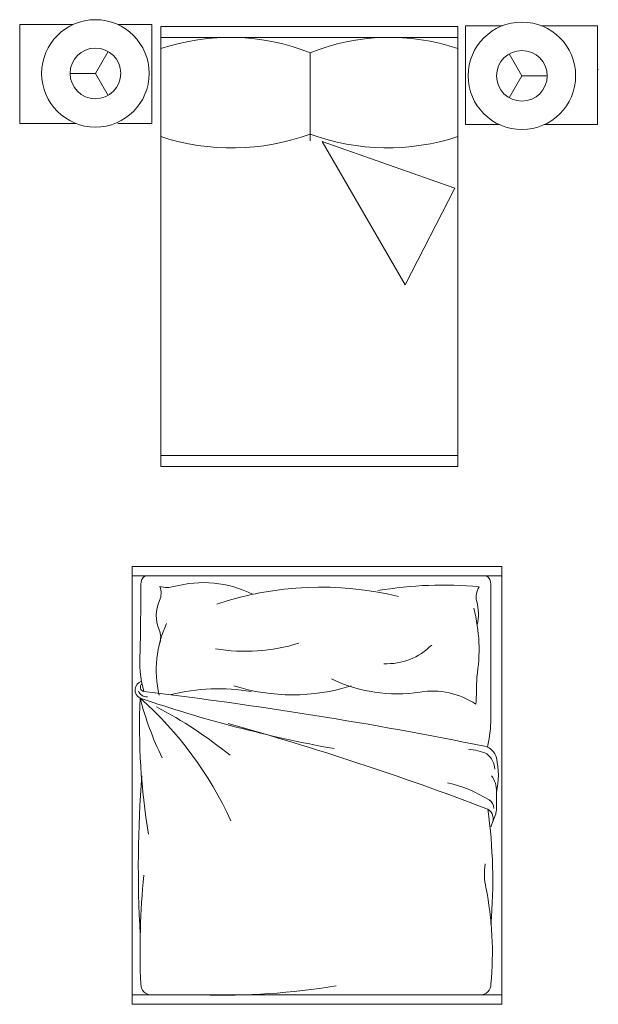
# Model space of a CAD drawing. Units: inches. Extents: x 1994 to 3075, y 3517 to 3950.
# Tile 10 of 58: x 1994.1175 to 1994.221, y 3553.7079 to 3553.8842. Entities that reach past the tile are written whole.
import ezdxf

# ---------------------------------------------------------------- set-up
doc = ezdxf.new("R2010")
doc.units = ezdxf.units.IN
doc.layers.add('A-FURN-REFR', color=8, linetype='Continuous', lineweight=13)

msp = doc.modelspace()

# ---------------------------------------------------------------- linework, layer by layer
at = {"layer": 'A-FURN-REFR'}
for p, q in [((1994.117509432348, 3553.883333005121), (1994.117509432348, 3553.865616469688)), ((1994.127049437094, 3553.883333005121), (1994.117509432348, 3553.883333005121)), ((1994.141131479592, 3553.883333005121), (1994.135063195254, 3553.883333005121)), ((1994.141131479592, 3553.883333005121), (1994.141131479592, 3553.865616469688)), ((1994.142742782828, 3553.804228108823), (1994.142742782828, 3553.882968266304)), ((1994.195892389127, 3553.882968266304), (1994.142742782828, 3553.882968266304)), ((1994.195892389127, 3553.804228108823), (1994.195892389127, 3553.882968266304)), ((1994.19728760273, 3553.865416846483), (1994.19728760273, 3553.883133381916)), ((1994.19728760273, 3553.883133381916), (1994.203900343284, 3553.883133381916)), ((1994.210825189012, 3553.883133381916), (1994.220909649974, 3553.883133381916)), ((1994.220909649974, 3553.865416846483), (1994.220909649974, 3553.883133381916)), ((1994.195892389127, 3553.880999762367), (1994.142742782828, 3553.880999762367)), ((1994.131056316174, 3553.874589508938), (1994.133323201859, 3553.878515870119)), ((1994.169474900446, 3553.862532974195), (1994.169474900446, 3553.878281005691)), ((1994.207362766148, 3553.874160342666), (1994.205095880463, 3553.878086703847)), ((1994.221034633952, 3553.875241371727), (1994.220909649974, 3553.875366355705)), ((1994.131056316174, 3553.874589508938), (1994.126522544804, 3553.874589508938)), ((1994.131056316174, 3553.874589508938), (1994.133323201859, 3553.870663147756)), ((1994.207362766148, 3553.874160342666), (1994.205095880463, 3553.870233981485)), ((1994.207362766148, 3553.874160342666), (1994.211896537518, 3553.874160342666)), ((1994.12759389331, 3553.865616469688), (1994.117509432348, 3553.865616469688)), ((1994.141131479592, 3553.865616469688), (1994.135063195254, 3553.865616469688)), ((1994.19728760273, 3553.865416846483), (1994.203355887068, 3553.865416846483)), ((1994.211369645228, 3553.865416846483), (1994.220909649974, 3553.865416846483)), ((1994.195360842532, 3553.854041419548), (1994.171645162721, 3553.862373044578)), ((1994.186492509023, 3553.836735927227), (1994.171645162721, 3553.862373044578)), ((1994.195360842532, 3553.854041419548), (1994.186492509023, 3553.836735927227)), ((1994.195892389127, 3553.80619661276), (1994.142742782828, 3553.80619661276)), ((1994.195892389127, 3553.804228108823), (1994.142742782828, 3553.804228108823)), ((1994.13761850143, 3553.786327657019), (1994.203768317831, 3553.786327657006)), ((1994.13761850143, 3553.786327657019), (1994.137618501414, 3553.707920668756)), ((1994.203768317831, 3553.786327657006), (1994.203768317815, 3553.707920668742)), ((1994.137618501429, 3553.784654455781), (1994.20376831783, 3553.784654455768)), ((1994.20182273499, 3553.759147087566), (1994.201822734995, 3553.783097989499)), ((1994.202795526404, 3553.742699450552), (1994.202795526405, 3553.746517277539)), ((1994.202675320726, 3553.742026181805), (1994.201822734986, 3553.739714637505)), ((1994.137618501414, 3553.709593869994), (1994.203768317815, 3553.709593869981)), ((1994.137618501414, 3553.707920668756), (1994.203768317815, 3553.707920668742))]:
    msp.add_line(p, q, dxfattribs=at)
for centre, radius in [((1994.131056316174, 3553.874589508938), 0.0096178898656984), ((1994.207362766148, 3553.874160342666), 0.0096178898656984), ((1994.131056316174, 3553.874589508938), 0.004533771369707), ((1994.207362766148, 3553.874160342666), 0.004533771369707)]:
    msp.add_circle(centre, radius, dxfattribs=at)
for centre, radius, start, end in [((1994.155078837424, 3553.84195624103), 0.0390734584879713, 68.38081539171897, 108.4039485392068), ((1994.183695872419, 3553.843014126873), 0.0380261592246056, 71.29230697710972, 111.9612016907544), ((1994.15550083672, 3553.902282602643), 0.0410331481229022, 251.8852769299205, 289.9107209210493), ((1994.183286182339, 3553.901481352651), 0.0402245355213375, 249.9186093217453, 288.2640062866705), ((1994.141120550532, 3553.783097989512), 0.0019455828353276, 126.8698976337993, 179.9999999880876), ((1994.19987715216, 3553.7830979895), 0.0019455828353276, 359.9999999880876, 53.13010234330246), ((1993.601556575717, 3553.782256987198), 0.5376190497749752, 358.8114973710085, 0.0896283401223897), ((1994.139610526882, 3553.781527333681), 0.0032028341489732, 335.7877323280015, 21.71237864400314), ((1994.143846681053, 3553.787202677152), 0.0046640380554646, 254.3196277006035, 285.6803722997152), ((1994.1503379227, 3553.763668816497), 0.0197486987265365, 63.38196750841395, 105.3587807882128), ((1994.171396254335, 3553.723937389351), 0.0586716085832465, 76.33335198625635, 108.4694926903225), ((1994.193173667668, 3553.714879910245), 0.0680947404926167, 84.45870901972506, 99.7951687550354), ((1994.202275155399, 3553.780846544132), 0.0031075126812102, 144.3787648229011, 195.1987658355305), ((1994.148529566308, 3553.777516662834), 0.0065764677133891, 155.7877323280015, 202.8808293159797), ((1994.169841135078, 3553.771464333994), 0.0298558147000044, 350.3711224665587, 14.25995084780135), ((1994.190980737527, 3553.777778179954), 0.0085962787467616, 347.311957921453, 15.19876583553051), ((1994.161796708111, 3553.767753433195), 0.0198519972069101, 155.1179531461462, 192.9861889591517), ((1994.139393198019, 3553.773660911681), 0.0033401870886801, 339.0160855821216, 22.88082931597971), ((1994.15788917563, 3553.803354051666), 0.0322267158934928, 260.4320326468418, 287.2701993260345), ((1994.183123582284, 3553.780345114184), 0.0114567055564695, 267.8294752673963, 315.0098308273483), ((1994.159032850035, 3553.769377849948), 0.0200474922626186, 175.0553728283678, 195.8557099358243), ((1994.185028245591, 3553.790544852875), 0.0270339202009644, 244.2263214075132, 278.7465115985381), ((1994.130857860752, 3553.766249810661), 0.0684188319639238, 356.1489785764833, 0.1847956127646253), ((1994.139768127038, 3553.764205594758), 0.0016105685091622, 106.3004786234319, 243.938180591863), ((1994.139915374633, 3553.764696054451), 0.0008128892221172, 129.3957755051945, 258.1255955891823), ((1994.153014092121, 3553.729829161485), 0.034582210914614, 80.14382640862489, 104.1008515969175), ((1994.166331785783, 3553.798564028057), 0.0352368026282888, 252.6579936860071, 287.3420063136771), ((1994.140236130078, 3553.764592074247), 0.0016095821071006, 202.6051908922757, 274.4988817166678), ((1994.255577321717, 3553.757659476503), 0.1166283141987217, 177.4940716817132, 189.5094068679036), ((1994.095590157615, 3553.713705169825), 0.065543355857517, 24.38326925012849, 48.45324971012612), ((1994.215796953557, 3553.985577945495), 0.2356625857026807, 250.9968676421653, 259.7279623061984), ((1994.191499669869, 3553.776017591432), 0.0540893550839264, 194.1893851607317, 206.3095844034524), ((1994.053303561478, 3553.031122886954), 0.737858914858732, 78.47703152821846, 83.27200853442297), ((1994.191370939103, 3553.750047845144), 0.0139570689006921, 56.2641403896707, 99.20148074358214), ((1994.103609109213, 3553.688779030386), 0.0819509525067612, 51.03759283326017, 62.08562985249065), ((1994.177105438502, 3553.75947872609), 0.0247195212287987, 347.0890423172248, 359.2312934508153), ((1994.011503619994, 3553.244683136573), 0.5331120127502642, 69.18683318772709, 74.4079909335134), ((1994.20015049773, 3553.751441980071), 0.0027238159694586, 12.88269036848606, 78.38686031445394), ((1994.197260249739, 3553.744471056852), 0.0091331594194461, 65.03385580996276, 86.4640048798947), ((1994.198613258533, 3553.749705051654), 0.0039416012902181, 4.684898432501862, 50.59840531545589), ((1994.189325642241, 3553.748966198805), 0.013828183994568, 346.9286456497866, 12.88269036848606), ((1994.355546155189, 3553.732585489288), 0.2168115609509192, 175.697202442643, 183.2229785434103), ((1994.198608338384, 3553.746268636669), 0.0041945638393764, 356.601689895136, 37.73019638534235), ((1994.18847503089, 3553.723661673473), 0.0245737753138132, 58.01122975656369, 76.86512646864662), ((1994.200610557941, 3553.743017802381), 0.001728440251783, 359.0101027185217, 59.29760239232226), ((1994.200286002193, 3553.741170483539), 0.0019455828353276, 339.7541012352643, 70.67241641354788), ((1994.108974103747, 3553.730077626183), 0.0931787946855045, 355.1752823324409, 7.876466900264919), ((1994.200849943569, 3553.742699450552), 0.0019455828353276, 339.7541012352643, 359.9999999880876), ((1994.200849943569, 3553.742699450552), 0.0019455828353276, 339.7541012352643, 359.9999999880876), ((1994.213641877956, 3553.731364013998), 0.0129749866847535, 172.4746658505032, 191.3425348756069), ((1994.280338002942, 3553.717521347986), 0.1412897221787423, 174.5126540947314, 182.4265021931356), ((1994.142543710628, 3553.717102301263), 0.0595394659951302, 354.6389628949611, 11.34253487560691), ((1994.141120550518, 3553.711539452829), 0.0019455828353276, 179.9999999880876, 269.9999999880876), ((1994.199877152144, 3553.711539452816), 0.0019455828353276, 269.9999999880876, 359.9999999880876), ((1994.153663027019, 3553.833679777337), 0.1241401229318277, 268.3066004926072, 279.4831521227457)]:
    msp.add_arc(centre, radius, start, end, dxfattribs=at)

doc.saveas('drawing.dxf')
